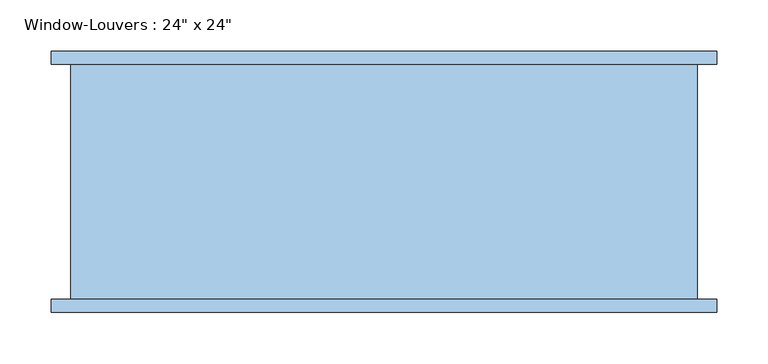
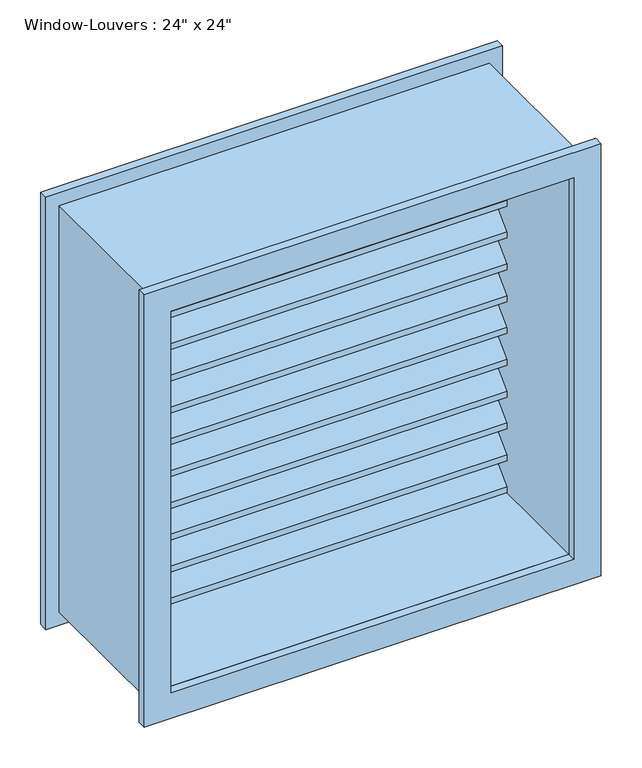
"""IFC4 building model written with IfcOpenShell, lengths in millimetres: window geometry."""

from ifc_helpers import new_model, si_unit, frame, origin, place, context, project, spatial, polyline, outline, extrude, source, transform, mapped, element, save


def window_f2d8fef0(model_context):
    return source(origin(), model_context, "Body", "SweptSolid", [
        extrude(outline(polyline([(107.95, 1419.1754778), (107.95, 1410.1952217), (69.85, 1448.2952217), (31.75, 1410.1952217), (31.75, 1419.1754778), (69.85, 1457.2754778), (107.95, 1419.1754778)])), frame((-285.75, 0.0, 0.0), z_axis=(1.0, 0.0, 0.0), x_axis=(0.0, 1.0, 0.0)), (0.0, 0.0, 1.0), 571.5),
        extrude(outline(polyline([(107.95, 1371.5009557), (107.95, 1362.5206995), (69.85, 1400.6206995), (31.75, 1362.5206995), (31.75, 1371.5009557), (69.85, 1409.6009557), (107.95, 1371.5009557)])), frame((-285.75, 0.0, 0.0), z_axis=(1.0, 0.0, 0.0), x_axis=(0.0, 1.0, 0.0)), (0.0, 0.0, 1.0), 571.5),
        extrude(outline(polyline([(107.95, 1323.8264335), (107.95, 1314.8461774), (69.85, 1352.9461774), (31.75, 1314.8461774), (31.75, 1323.8264335), (69.85, 1361.9264335), (107.95, 1323.8264335)])), frame((-285.75, 0.0, 0.0), z_axis=(1.0, 0.0, 0.0), x_axis=(0.0, 1.0, 0.0)), (0.0, 0.0, 1.0), 571.5),
        extrude(outline(polyline([(107.95, 1276.1519113), (107.95, 1267.1716552), (69.85, 1305.2716552), (31.75, 1267.1716552), (31.75, 1276.1519113), (69.85, 1314.2519113), (107.95, 1276.1519113)])), frame((-285.75, 0.0, 0.0), z_axis=(1.0, 0.0, 0.0), x_axis=(0.0, 1.0, 0.0)), (0.0, 0.0, 1.0), 571.5),
        extrude(outline(polyline([(107.95, 1228.4773891), (107.95, 1219.497133), (69.85, 1257.597133), (31.75, 1219.497133), (31.75, 1228.4773891), (69.85, 1266.5773891), (107.95, 1228.4773891)])), frame((-285.75, 0.0, 0.0), z_axis=(1.0, 0.0, 0.0), x_axis=(0.0, 1.0, 0.0)), (0.0, 0.0, 1.0), 571.5),
        extrude(outline(polyline([(107.95, 1180.802867), (107.95, 1171.8226109), (69.85, 1209.9226109), (31.75, 1171.8226109), (31.75, 1180.802867), (69.85, 1218.902867), (107.95, 1180.802867)])), frame((-285.75, 0.0, 0.0), z_axis=(1.0, 0.0, 0.0), x_axis=(0.0, 1.0, 0.0)), (0.0, 0.0, 1.0), 571.5),
        extrude(outline(polyline([(107.95, 1133.1283448), (107.95, 1124.1480887), (69.85, 1162.2480887), (31.75, 1124.1480887), (31.75, 1133.1283448), (69.85, 1171.2283448), (107.95, 1133.1283448)])), frame((-285.75, 0.0, 0.0), z_axis=(1.0, 0.0, 0.0), x_axis=(0.0, 1.0, 0.0)), (0.0, 0.0, 1.0), 571.5),
        extrude(outline(polyline([(107.95, 1085.4538226), (107.95, 1076.4735665), (69.85, 1114.5735665), (31.75, 1076.4735665), (31.75, 1085.4538226), (69.85, 1123.5538226), (107.95, 1085.4538226)])), frame((-285.75, 0.0, 0.0), z_axis=(1.0, 0.0, 0.0), x_axis=(0.0, 1.0, 0.0)), (0.0, 0.0, 1.0), 571.5),
        extrude(outline(polyline([(107.95, 1037.7793005), (107.95, 1028.7990443), (69.85, 1066.8990443), (31.75, 1028.7990443), (31.75, 1037.7793005), (69.85, 1075.8793005), (107.95, 1037.7793005)])), frame((-285.75, 0.0, 0.0), z_axis=(1.0, 0.0, 0.0), x_axis=(0.0, 1.0, 0.0)), (0.0, 0.0, 1.0), 571.5),
        extrude(outline(polyline([(107.95, 990.1047783), (107.95, 981.1245222), (69.85, 1019.2245222), (31.75, 981.1245222), (31.75, 990.1047783), (69.85, 1028.2047783), (107.95, 990.1047783)])), frame((-285.75, 0.0, 0.0), z_axis=(1.0, 0.0, 0.0), x_axis=(0.0, 1.0, 0.0)), (0.0, 0.0, 1.0), 571.5),
        extrude(outline(polyline([(107.95, 1466.85), (107.95, 1457.8697439), (69.85, 1495.9697439), (31.75, 1457.8697439), (31.75, 1466.85), (69.85, 1504.95), (107.95, 1466.85)])), frame((-285.75, 0.0, 0.0), z_axis=(1.0, 0.0, 0.0), x_axis=(0.0, 1.0, 0.0)), (0.0, 0.0, 1.0), 571.5),
        extrude(outline(polyline([(107.95, 942.4302561), (107.95, 933.45), (69.85, 971.55), (31.75, 933.45), (31.75, 942.4302561), (69.85, 980.5302561), (107.95, 942.4302561)])), frame((-285.75, 0.0, 0.0), z_axis=(1.0, 0.0, 0.0), x_axis=(0.0, 1.0, 0.0)), (0.0, 0.0, 1.0), 571.5),
        extrude(outline(polyline([(1524.0, 304.8), (1524.0, -304.8), (914.4, -304.8), (914.4, 304.8), (1524.0, 304.8)]), holes=[polyline([(1504.95, 285.75), (933.45, 285.75), (933.45, -285.75), (1504.95, -285.75), (1504.95, 285.75)])]), frame((0.0, -120.65, 0.0), z_axis=(0.0, 1.0, 0.0), x_axis=(0.0, 0.0, 1.0)), (0.0, 0.0, 1.0), 228.6),
        extrude(outline(polyline([(1543.05, 323.85), (1543.05, -323.85), (895.35, -323.85), (895.35, 323.85), (1543.05, 323.85)]), holes=[polyline([(1504.95, 285.75), (933.45, 285.75), (933.45, -285.75), (1504.95, -285.75), (1504.95, 285.75)])]), frame((0.0, -133.35, 0.0), z_axis=(0.0, 1.0, 0.0), x_axis=(0.0, 0.0, 1.0)), (0.0, 0.0, 1.0), 12.7),
        extrude(outline(polyline([(1543.05, -323.85), (895.35, -323.85), (895.35, 323.85), (1543.05, 323.85), (1543.05, -323.85)]), holes=[polyline([(1504.95, -285.75), (1504.95, 285.75), (933.45, 285.75), (933.45, -285.75), (1504.95, -285.75)])]), frame((0.0, 107.95, 0.0), z_axis=(0.0, 1.0, 0.0), x_axis=(0.0, 0.0, 1.0)), (0.0, 0.0, 1.0), 12.7),
    ])


if __name__ == "__main__":
    model = new_model("IFC4")
    model_context = context("Model", 3, world=origin())
    ifc_project = project(units=[si_unit("LENGTHUNIT", "METRE", prefix="MILLI")], contexts=[model_context])
    site = spatial("IfcSite", under=ifc_project)
    building = spatial("IfcBuilding", under=site)
    placement = place(None, origin())
    window_shape = window_f2d8fef0(model_context)
    element("IfcWindow", 1, ObjectType="Window-Louvers : 24\" x 24\"", at=placement, inside=building, context=model_context, shape_type="MappedRepresentation", body=[
        mapped(window_shape, transform((0.0, 0.0, 0.0), x_axis=(1.0, 0.0, 0.0), y_axis=(0.0, 1.0, 0.0), z_axis=(0.0, 0.0, 1.0))),
    ])
    save(model, "model.ifc")

# Revit data of these elements
# Type "Window-Louvers : 24\" x 24\""
#   Type Mark = "20"
#   Construction Type Id = "GSP4R"
#   Assembly Code = "B20"
#   Analytic Construction = "1/8 in Pilkington single glazing"
#   Visual Light Transmittance = 0.9
#   Thermal Resistance (R) = 1.53941 (h·ft²·°F)/BTU
#   Solar Heat Gain Coefficient = 0.78
#   Max Height = 1' - 11.74264"
#   Height = 2' - 0"
#   Heat Transfer Coefficient (U) = 0.6496 BTU/(h·ft²·°F)
#   Blade Width [instance default] = 1' - 10 1/2"
#   Blade Vertical Thickness = 0' - 0.35355"
#   Blade Thickness = 0' - 0 1/4"
#   Blade Spacing = 0' - 1 1/2"
#   Blade Height = 0' - 1.85355"
#   Blade Depth = 0' - 3"
#   Blade Angle = 45.00°
#   Default Sill Height = 3' - 0"
#   Trim Projection_Exterior = 0' - 0 1/2"
#   Trim Projection_Interior = 0' - 0 1/2"
#   Trim Width_Exterior = 0' - 1 1/2"
#   Trim Width_Interior = 0' - 1 1/2"
#   Width = 2' - 0"
#   Max Blade Count = 12
#   Define Thermal Properties by = 1
#   Blade Count = 12
#   Frame Material = Birch
#   Louver Material = Birch
#   Trim Exterior Material = Birch
#   Trim Interior Material = Birch
#   Wall Closure = (empty or 0)
# Element 1 (IfcWindow, "Window-Louvers : 24\" x 24\"")
#   Materials on its faces: "Birch"
# Materials
#   "Birch": class "Wood", colour RGB 224 178 126, transparency 0, Description = "Betula Alleghaniensis", Cost = 0
